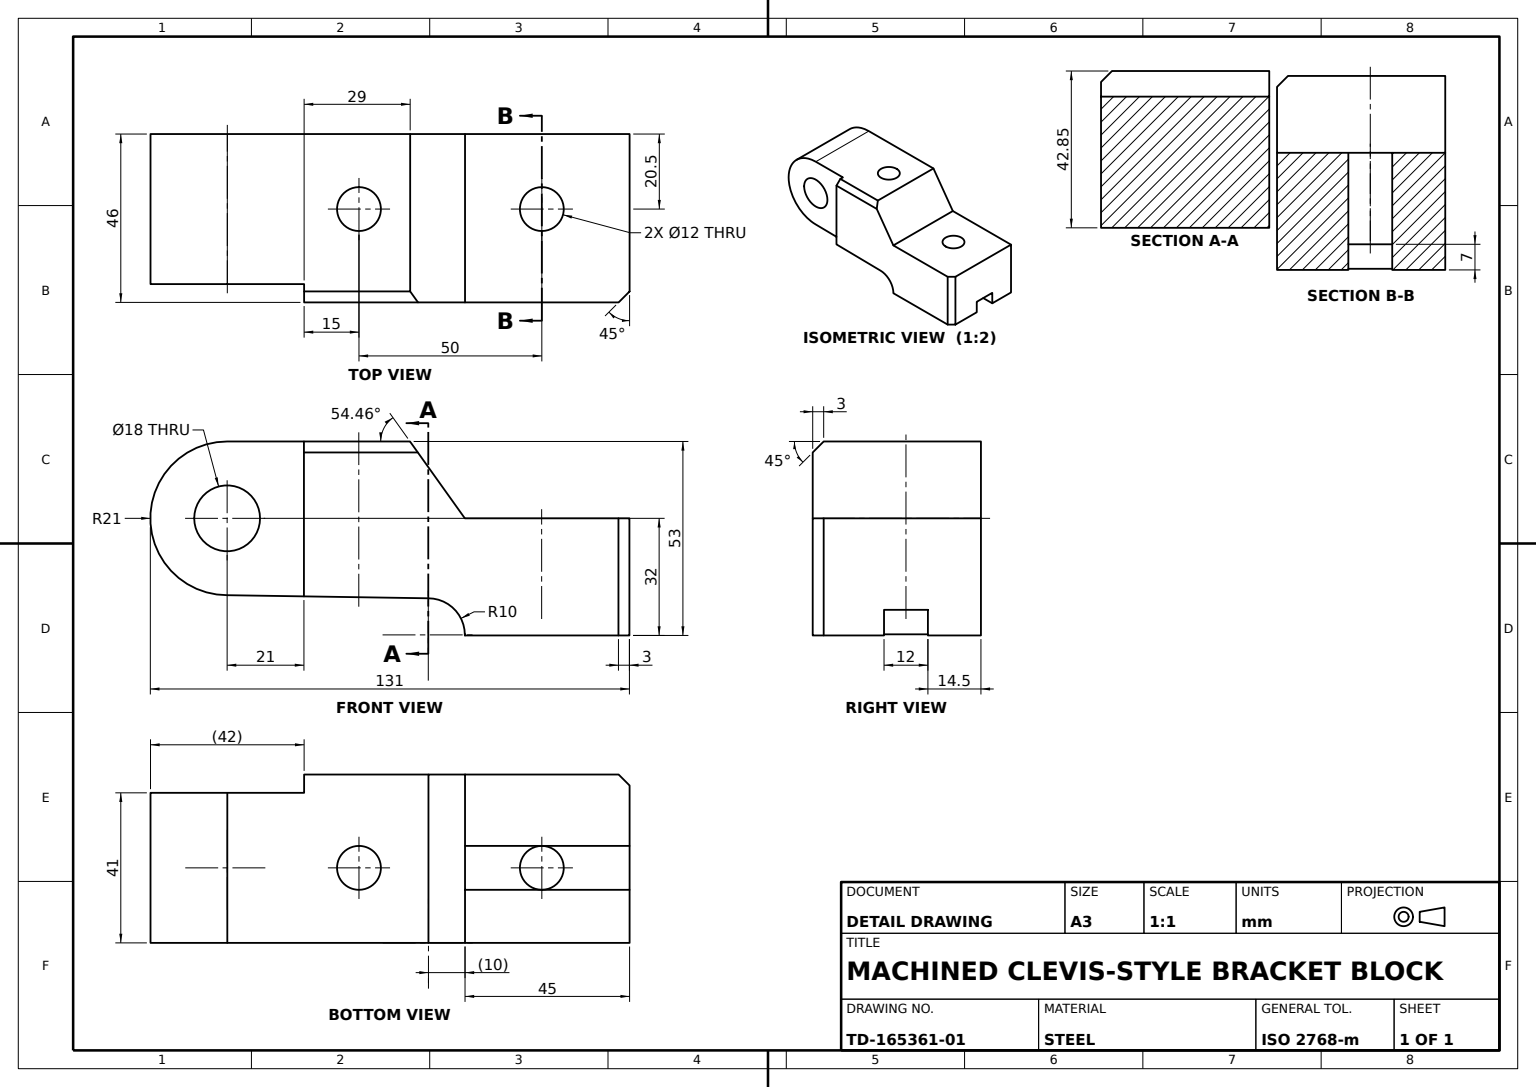
SolidWorks part; units mm, degrees
material "Plain Carbon Steel"
ref_plane "Front Plane" through (0, 0, 0) normal (0, 0, 1) x (1, 0, 0)
ref_plane "Top Plane" through (0, 0, 0) normal (0, 1, 0) x (1, 0, 0)
ref_plane "Right Plane" through (0, 0, 0) normal (1, 0, 0) x (0, 0, -1)
sketch "Base Block Profile" plane through (0, 0, 0) normal (0, 0, 1) x (1, 0, 0)
  line L0 (0, 0) -> (45, 0)
  line L1 (45, 0) -> (45, -32)
  line L2 (45, -32) -> (0, -32)
  line L3 (0, 0) -> (0, -32)
  dimension "D1" = 45
  dimension "D2" = 32
  dimension "D3" = 45
extrude "Base Block" add sketch "Base Block Profile" along normal blind 41
sketch "End Slot Profile" plane through (45, 0, 0) normal (1, 0, 0) x (0, 0, -1)
  line L0 (-26.5, -32) -> (-14.5, -32)
  line L1 (-41, -32) -> (0, -32) construction
  line L2 (-26.5, -32) -> (-26.5, -25)
  line L3 (-26.5, -25) -> (-14.5, -25)
  line L4 (-14.5, -25) -> (-14.5, -32)
  line L5 (0, -32) -> (0, 0) construction
  dimension "D1" = 14.5
  dimension "D2" = 7
  dimension "D3" = 12
extrude "End Slot 7x12" cut sketch "End Slot Profile" against normal blind 45
sketch "Arm Extension Profile" plane through (0, 0, 41) normal (0, 0, 1) x (1, 0, 0)
  line L0 (-65, 21) -> (-15, 21)
  line L2 (0, -32) -> (0, -31.6923)
  line L3 (0, 0) -> (0, -32) construction
  line L4 (-65, -21) -> (-9.6912, -21.8509)
  line L5 (0, 0) -> (0, -22)
  line L6 (-15, 21) -> (0, 0)
  line L7 (-9.6912, -21.8509) -> (-9.9988, -21.8462)
  arc A0 (-65, 21) -> (-65, -21) centre (-65, 0) ccw
  arc A1 (0, -32) -> (-9.9988, -21.8462) centre (-9.9988, -31.8462) ccw
  line M1 (0, 0) -> (0, -32)
  dimension "D3" = 21
  dimension "D4" = 10
  dimension "D6" = 21
  dimension "D1" = 50
  dimension "D2" = 10
  dimension "D5" = 10
  dimension "D7" = 15
  dimension "D8" = 42.8462
extrude "Arm Extension" add sketch "Arm Extension Profile" against normal blind 41 contours A1 L6 L0 A0 L4 M1
sketch "Underside Relief Profile" plane through (0, 21, 0) normal (0, 1, 0) x (1, 0, 0)
  line L1 (-86, -41) -> (-44, -41)
  line L2 (-65, -41) -> (-15, -41) construction
  circle A0 centre (-29, -20.5) radius 6
  circle A1 centre (21, -20.5) radius 6
  dimension "D1" = 6
  dimension "D5" = 6
  dimension "D2" = 15
  dimension "D3" = 42
  dimension "D4" = 50
  dimension "D6" = 20.5
extrude "Underside Relief Cut" cut sketch "Underside Relief Profile" against normal blind 50 contours A0 | A1
sketch "Raised Pad Profile" plane through (0, 0, 41) normal (0, 0, 1) x (1, 0, 0)
  line L0 (-86, 0) -> (-44, 0)
  line L1 (-44, 0) -> (-44, 21)
  line L2 (-44, 0) -> (-44, -21.3231)
  line L3 (-15, 21) -> (-44, 21)
  line L5 (-9.9988, -21.8462) -> (-44, -21.3231)
  line L7 (0, -32) -> (45, -32)
  line L8 (45, -32) -> (45, 0)
  line L9 (45, 0) -> (0, 0)
  arc A0 (-65, 21) -> (-65, -21) centre (-65, 0) ccw construction
  arc A1 (-9.9988, -21.8462) -> (0, -32) centre (-9.9988, -31.8462) cw
  line M4 (45, 0) -> (0, 0)
  line M5 (0, 0) -> (-15, 21)
  line M6 (-15, 21) -> (-65, 21)
  line M8 (-65, -21) -> (-9.9988, -21.8462)
  arc M9 (-9.9988, -21.8462) -> (0, -31.6923) centre (-9.9988, -31.8462) cw
  line M11 (0, -32) -> (45, -32)
  line M12 (45, -32) -> (45, 0)
  dimension "D2" = 10
  dimension "D1" = 42
  dimension "D3" = 29
  dimension "D4" = 20.6745
extrude "Raised Pad" add sketch "Raised Pad Profile" along normal blind 5 contours A1 L1 L2 M9 M11 M12 M4 M5 M6 M8
sketch "Pivot Bore Profile" plane through (0, 0, 41) normal (0, 0, 1) x (1, 0, 0)
  circle A0 centre (-65, 0) radius 9
  dimension "D1" = 18
extrude "Pivot Bore Ø18" cut sketch "Pivot Bore Profile" against normal blind 50
chamfer "Pad Chamfer 3x45 A" distance 3 angle 45 1 edges at (-29.5, 21, 46)
chamfer "Pad Chamfer 3x45 B" distance 3 angle 45 1 edges at (45, -16, 46)
